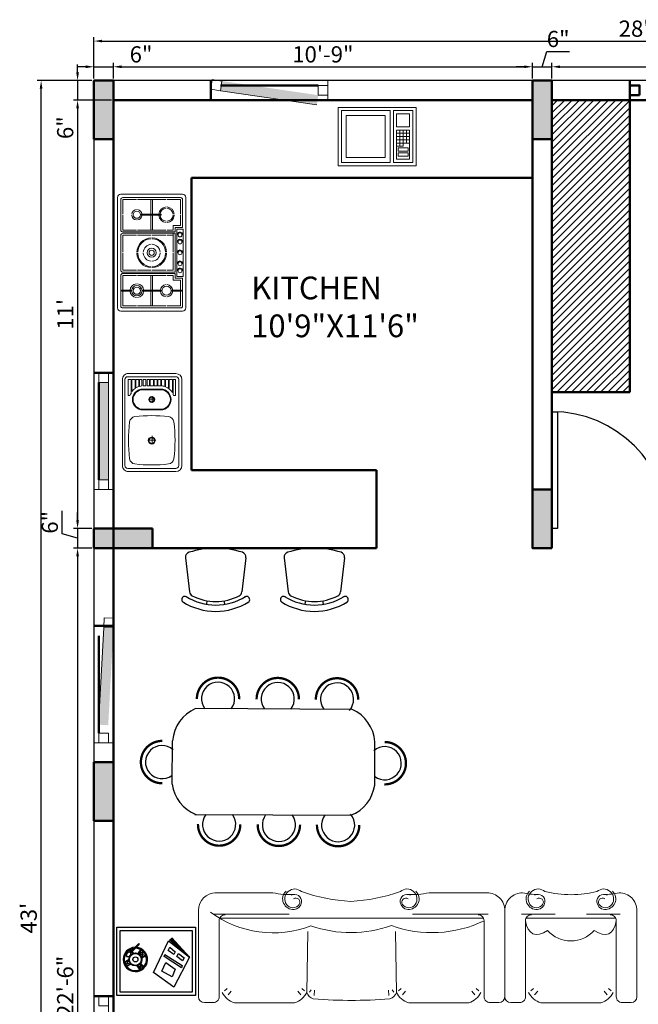
# Model space of a CAD drawing. Units: inches. Extents: x 3064 to 19385, y 846 to 15425.
# Tile 58 of 108: x 6020 to 6210, y 1703 to 2007. Entities that reach past the tile are written whole.
import ezdxf

# ---------------------------------------------------------------- set-up
doc = ezdxf.new("R2010")
doc.units = ezdxf.units.IN
for name, color, linetype, lineweight in [('A-ANNO-DIMS', 2, 'Continuous', 18), ('A-AREA-IDEN', 3, 'Continuous', 18), ('A-COLS', 1, 'Continuous', 35), ('A-DOOR', 3, 'Continuous', 25), ('A-EQPM', 8, 'Continuous', 18), ('A-FLOR-FIXT', 9, 'Continuous', 18), ('A-FURN', 8, 'Continuous', 18), ('A-FURN-PATT', 252, 'Continuous', 13), ('A-GLAZ', 4, 'Continuous', 18), ('A-WALL', 7, 'Continuous', 50), ('C-PROP', 6, 'Continuous', 25)]:
    doc.layers.add(name, color=color, linetype=linetype, lineweight=lineweight)
for name, color, linetype in [('BLO', 135, 'Continuous'), ('FUR', 42, 'Continuous'), ('NOITHAT', 21, 'Continuous'), ('Win', 152, 'Continuous')]:
    doc.layers.add(name, color=color, linetype=linetype)
doc.styles.get("Standard").update_dxf_attribs({"font": 'arial.ttf'})
doc.dimstyles.new('ISO-25', dxfattribs={"dimtxt": 9, "dimasz": 2.5, "dimexe": 1.25, "dimexo": 0.625, "dimtad": 1, "dimdec": 1, "dimlunit": 3, "dimtxsty": 'Standard', "dimcen": 2.5, "dimadec": 0, "dimazin": 0, "dimtfac": 1, "dimtdec": 1, "dimtmove": 0, "dimatfit": 3, "dimfxl": 1, "dimarcsym": 0})

# ---------------------------------------------------------------- blocks, each defined once
blk = doc.blocks.new('*U3')
for p, q in [((0, 0), (0, -6)), ((36, 0), (36, -6))]:
    blk.add_line(p, q)
blk.add_lwpolyline([(0, 0), (0, 36), (1.75, 36), (1.75, 0)], close=True)
blk.add_arc((0, 0), 36, 0, 90)
blk = doc.blocks.new('din')
at = {"layer": 'FUR', "ltscale": 0.25}
for p, q in [((70.23, 15.24), (9.28, 15.24)), ((0, 3.44), (0, -13.56)), ((79.14, 3.44), (79.14, -13.56)), ((8.91, -26.16), (70.23, -26.16))]:
    blk.add_line(p, q, dxfattribs=at)
at = {"layer": 'FUR', "ltscale": 0.25, "const_width": 0.9}
for points in [[(22.5, 19.02, 1.012537), (5.94, 19.02, 1.012537)], [(45.67, 19.02, 1.012537), (29.11, 19.02, 1.012537)], [(69.02, 19.02, 1.012537), (52.46, 19.02, 1.012537)], [(-3.79, 3.1, 1.012537), (-3.79, -13.47, 1.012537)], [(83.08, 3.1, -1.012537), (83.08, -13.47, -1.012537)], [(23.18, -29.95, -1.012537), (6.61, -29.95, -1.012537)], [(46.34, -29.95, -1.012537), (29.78, -29.95, -1.012537)], [(69.7, -29.95, -1.012537), (53.14, -29.95, -1.012537)]]:
    blk.add_lwpolyline(points, format="xyb", dxfattribs=at)
at = {"layer": 'FUR', "ltscale": 0.25}
for centre, radius, start, end in [((14.22, 19.13), 6.48, 323.1301, 221.2163), ((37.39, 19.13), 6.48, 323.1301, 216.8699), ((60.74, 19.13), 6.48, 323.1301, 216.8699), ((14.55, 1.54), 14.67, 111.0491, 172.5731), ((64.59, 1.54), 14.67, 7.4269, 68.9509), ((-3.89, -5.18), 6.48, 53.1301, 311.2163), ((83.18, -5.18), 6.48, 228.7837, 126.8699), ((15.28, -12.21), 15.34, 185.0602, 245.4675), ((63.86, -12.21), 15.34, 294.5325, 354.9398), ((14.89, -30.05), 6.48, 138.7837, 36.8699), ((38.06, -30.05), 6.48, 143.1301, 36.8699), ((61.42, -30.05), 6.48, 143.1301, 36.8699)]:
    blk.add_arc(centre, radius, start, end, dxfattribs=at)
blk = doc.blocks.new('A$C558E769F')
at = {"layer": 'NOITHAT'}
for p, q in [((29.4, 426.4), (61.1, 154.1)), ((508.9, 426.4), (477.2, 154.1)), ((197.1, 55.9), (201.8, 84.2)), ((341.2, 55.9), (336.5, 84.2))]:
    blk.add_line(p, q, dxfattribs=at)
for centre, radius, start, end in [((69.1, 431), 40, 107.02981, 186.63805), ((269.2, -222), 723, 72.97019, 107.02981), ((469.2, 431), 40, 353.36195, 72.97019), ((25.3, 93.7), 25.7, 44.80366, 252.32262), ((269.2, 492.6), 442.6, 237.77056, 302.22944), ((100.8, 158.7), 40, 186.63805, 243.24485), ((269.2, 492.6), 413.9, 243.24485, 296.75515), ((437.5, 158.7), 40, 296.75515, 353.36195), ((513, 93.7), 25.7, 287.67738, 135.19634), ((269.2, 492.6), 492.6, 237.85101, 302.14899)]:
    blk.add_arc(centre, radius, start, end, dxfattribs=at)
blk = doc.blocks.new('sofa-32')
at = {"color": 0, "linetype": 'ByBlock'}
for p, q in [((-0.026, 0.9238), (-0.1, 0.9238)), ((0.657, 0.9252), (0.1531, 0.9252)), ((1.6158, 0.9252), (2.1197, 0.9252)), ((2.3728, 0.9238), (2.2988, 0.9238)), ((-0.15, 0.15), (-0.15, 0.8738)), ((0.024, 0.2361), (0.024, 0.8738)), ((0.05, 0.8375), (0.05, 0.8379)), ((0.1006, 0.8574), (0.1265, 0.8286)), ((0.7096, 0.8574), (0.6837, 0.8286)), ((0.7682, 0.3257), (0.7597, 0.8384)), ((0.7601, 0.8375), (0.7601, 0.8379)), ((0.7823, 0.8346), (0.7966, 0.8162)), ((0.8227, 0.8633), (0.8259, 0.8195)), ((1.4501, 0.8633), (1.447, 0.8195)), ((1.4906, 0.8346), (1.4762, 0.8162)), ((1.5046, 0.3257), (1.5131, 0.8384)), ((1.5127, 0.8375), (1.5127, 0.8379)), ((1.5632, 0.8574), (1.5891, 0.8286)), ((2.1722, 0.8574), (2.1463, 0.8286)), ((2.2228, 0.8375), (2.2228, 0.8379)), ((2.2228, 0.8375), (2.2228, 0.8379)), ((2.2488, 0.2361), (2.2488, 0.8738)), ((2.4228, 0.15), (2.4228, 0.8738)), ((0.0903, 0.8062), (0.0682, 0.8242)), ((0.7199, 0.8062), (0.742, 0.8242)), ((1.5529, 0.8062), (1.5308, 0.8242)), ((2.1825, 0.8062), (2.2046, 0.8242)), ((-0.01, 0.1801), (0.6238, 0.1801)), ((0.0289, 0.2145), (2.2439, 0.2145)), ((2.2948, 0.1801), (1.661, 0.1801)), ((0, 0), (0.4856, 0)), ((2.2848, 0), (1.7991, 0))]:
    blk.add_line(p, q, dxfattribs=at)
at = {"color": 0, "linetype": 'ByBlock', "extrusion": (0, 0, -1)}
for centre, major_axis, start_param, end_param in [((-0.1, 0.8738), (0.0354, 0.0354), 3.926992, 5.497787), ((-0.026, 0.8738), (-0.0354, 0.0354), 0.785398, 2.356196), ((0.1997, 0.7661), (0.1173, 0.1173), 4.372209, 5.213218), ((0.6105, 0.7661), (0.1173, 0.1173), -0.500829, 0.34018), ((1.6624, 0.7661), (0.1173, 0.1173), 4.372209, 5.213218), ((2.0731, 0.7661), (-0.1173, 0.1173), 1.069968, 1.910976), ((2.2988, 0.8738), (-0.0354, 0.0354), 5.497786, 7.068583), ((2.3728, 0.8738), (0.0354, 0.0354), -0.785398, 0.785398), ((0.8378, 0.8143), (-0.0573, 0.0573), 5.78837, 6.779907), ((1.1202, -2.7856), (2.6094, 2.6094), -0.86827, -0.778364), ((1.1526, -2.7856), (2.6094, 2.6094), -0.792432, -0.702526), ((1.435, 0.8143), (-0.0573, 0.0573), 1.074075, 2.065611), ((0.4599, -0.6685), (0.71, 0.71), 5.048761, 5.844539), ((1.1424, -0.6685), (-0.71, 0.71), 0.438646, 1.125824), ((1.7954, -0.5466), (-0.6249, 0.6249), 0.417642, 1.423136), ((0.074, 0.2361), (0.0354, 0.0354), 2.356194, 3.926992), ((2.1988, 0.2361), (0.0354, 0.0354), 0.785397, 2.356194), ((0, 0.15), (0.1061, 0.1061), 2.356194, 3.926992), ((0.6576, 0.0525), (-0.0624, 0.0624), 4.675944, 7.152385), ((0.6708, 0.0524), (-0.059, 0.059), 3.186406, 6.094039), ((0.6552, 0.0629), (0.0458, 0.0458), 4.523242, 6.472337), ((0.6801, 0.0798), (-0.0245, 0.0245), 1.759948, 4.523241), ((0.6592, 0.0712), (-0.0491, 0.0491), 0.8692, 2.230507), ((1.6256, 0.0712), (-0.0491, 0.0491), 5.623477, 6.984784), ((1.614, 0.0524), (0.059, 0.059), 0.189149, 3.096782), ((1.6047, 0.0798), (0.0245, 0.0245), 1.759947, 4.52324), ((1.6295, 0.0629), (0.0458, 0.0458), 4.52324, 6.472335), ((1.6271, 0.0525), (-0.0624, 0.0624), 0.701599, 3.17804), ((2.2728, 0.15), (0.1061, 0.1061), 0.785398, 2.356194), ((0.6324, -0.6613), (-0.479, 0.479), 0.566947, 0.842011), ((0.6701, 0.0726), (0.0414, 0.0414), 0.659711, 2.852687), ((1.2153, -1.3904), (1.0359, 1.0359), 5.158011, 5.447964), ((1.0694, -1.3904), (1.0359, 1.0359), 5.547613, 5.837566), ((1.6147, 0.0726), (-0.0414, 0.0414), 3.430501, 5.623477), ((1.6523, -0.6613), (0.479, 0.479), 5.441177, 5.716241)]:
    blk.add_ellipse(centre, major_axis=major_axis, ratio=1, start_param=start_param, end_param=end_param, dxfattribs=at)
blk = doc.blocks.new('sofa-34')
at = {"color": 0, "linetype": 'ByBlock'}
for p, q in [((-0.026, 0.9238), (-0.1, 0.9238)), ((0.657, 0.9252), (0.1531, 0.9252)), ((0.8361, 0.9238), (0.9101, 0.9238)), ((-0.15, 0.15), (-0.15, 0.8738)), ((0.024, 0.2361), (0.024, 0.8738)), ((0.05, 0.8375), (0.05, 0.8379)), ((0.1006, 0.8574), (0.1265, 0.8286)), ((0.7096, 0.8574), (0.6837, 0.8286)), ((0.7601, 0.8375), (0.7601, 0.8379)), ((0.7602, 0.8375), (0.7601, 0.8379)), ((0.7861, 0.2361), (0.7861, 0.8738)), ((0.9601, 0.15), (0.9601, 0.8738)), ((0.0903, 0.8062), (0.0682, 0.8242)), ((0.7199, 0.8062), (0.742, 0.8242)), ((-0.01, 0.1801), (0.2738, 0.1801)), ((0.0289, 0.2145), (0.7812, 0.2145)), ((0.8201, 0.1801), (0.5364, 0.1801))]:
    blk.add_line(p, q, dxfattribs=at)
blk.add_arc((0.4051, 0.1479), 0.2579, 40.79835, 139.20165, dxfattribs=at)
at = {"color": 0, "linetype": 'ByBlock', "extrusion": (0, 0, -1)}
for centre, major_axis, ratio, start_param, end_param in [((-0.1, 0.8738), (0.0354, 0.0354), 1, 3.926992, 5.497787), ((-0.026, 0.8738), (-0.0354, 0.0354), 1, 0.785398, 2.356196), ((0.1997, 0.7661), (0.1173, 0.1173), 1, 4.372209, 5.213218), ((0.6105, 0.7661), (0.1173, 0.1173), 1, -0.500829, 0.34018), ((0.5004, -0.5869), (-0.4145, 0.931), 0.264583, -0.381915, 0.387685), ((0.074, 0.2361), (-0.0354, 0.0354), 1, 3.926991, 5.497788), ((0, 0.15), (0.1061, 0.1061), 1, 2.356194, 3.926992), ((0.1167, 0.0525), (-0.0624, 0.0624), 1, 4.675944, 7.152385), ((0.1299, 0.0524), (-0.059, 0.059), 1, 3.186406, 6.094039), ((0.1144, 0.0629), (-0.0458, 0.0458), 1, 6.094039, 8.043134), ((0.1392, 0.0798), (0.0245, 0.0245), 1, 0.189152, 2.952444), ((0.1183, 0.0712), (0.0491, 0.0491), 1, -0.701597, 0.659711), ((0.179, -0.6576), (-0.2506, 0.635), 0.885019, 0.124301, 0.339591), ((0.1292, 0.0726), (-0.0414, 0.0414), 1, 2.230507, 4.423483), ((0.3517, -0.5578), (0.7346, 0.1067), 0.76838, 4.597815, 5.20076)]:
    blk.add_ellipse(centre, major_axis=major_axis, ratio=ratio, start_param=start_param, end_param=end_param, dxfattribs=at)
at = {"color": 0, "linetype": 'ByBlock'}
for centre, major_axis, ratio, start_param, end_param in [((0.8361, 0.8738), (0.0354, 0.0354), 1, 0.785398, 2.356196), ((0.9101, 0.8738), (-0.0354, 0.0354), 1, 3.926992, 5.497787), ((0.3097, -0.5869), (0.4145, 0.931), 0.264583, -0.381915, 0.387685), ((0.7361, 0.2361), (0.0354, 0.0354), 1, 3.926991, 5.497788), ((0.6918, 0.0712), (-0.0491, 0.0491), 1, -0.701597, 0.659711), ((0.6802, 0.0524), (0.059, 0.059), 1, 3.186406, 6.094039), ((0.6709, 0.0798), (-0.0245, 0.0245), 1, 0.189152, 2.952444), ((0.6958, 0.0629), (0.0458, 0.0458), 1, 6.094039, 8.043134), ((0.6934, 0.0525), (0.0624, 0.0624), 1, 4.675944, 7.152385), ((0.8101, 0.15), (-0.1061, 0.1061), 1, 2.356194, 3.926992), ((0.6809, 0.0726), (0.0414, 0.0414), 1, 2.230507, 4.423483), ((0.6312, -0.6576), (0.2506, 0.635), 0.885019, 0.124301, 0.339591)]:
    blk.add_ellipse(centre, major_axis=major_axis, ratio=ratio, start_param=start_param, end_param=end_param, dxfattribs=at)
blk = doc.blocks.new('sink 1')
for points in [[(-7.34, 1.48), (-7.34, 22.73)], [(-6.56, 1.48), (-6.56, 22.73)], [(5.86, 24.22), (-5.86, 24.22)], [(6.01, 23.43), (-5.86, 23.43)], [(6.72, 1.48), (6.72, 22.73)], [(7.34, 1.48), (7.34, 22.73)], [(0, 15.39), (0, 17.42)], [(1.09, 16.48), (-0.94, 16.48)], [(-2.09, 8.99), (2.28, 8.99)], [(-2.09, 8.84), (2.28, 8.84)], [(-5.78, 5.39), (-5.78, 5.39)], [(-5.31, 5.39), (-5.31, 5.39)], [(-5.16, 4.92), (-5.16, 4.92)], [(0.78, 6.33), (-0.78, 6.33)], [(0, 5.55), (0, 7.26)], [(5.16, 4.92), (5.16, 4.92)], [(5.94, 5.39), (5.94, 5.39)], [(-5, 1.48), (-5, 4.69)], [(-5, 1.48), (-4.22, 1.48), (-4.22, 3.83)], [(-4.84, 4.45), (-4.84, 4.45)], [(-4.22, 3.83), (-4.22, 3.83)], [(-4.06, 1.48), (-4.06, 3.69)], [(-4.06, 1.48), (-3.28, 1.48), (-3.28, 3.27)], [(-3.91, 3.52), (-3.91, 3.52)], [(-3.28, 3.2), (-3.28, 3.2)], [(-3.12, 3.2), (-3.12, 3.2)], [(-2.34, 3.05), (-2.34, 3.05)], [(-2.19, 3.05), (-2.19, 3.05)], [(-2.09, 3.99), (2.28, 3.99)], [(-2.09, 3.84), (2.28, 3.84)], [(-1.41, 3.05), (-1.41, 3.05)], [(-1.25, 3.05), (-1.25, 3.05)], [(-0.47, 1.48), (-1.25, 1.48), (-1.25, 3.05), (-0.47, 3.05)], [(-0.62, 3.05), (-0.62, 3.05)], [(-0.47, 1.48), (-0.47, 3.05)], [(-0.31, 3.05), (-0.31, 3.05)], [(0.47, 1.48), (-0.31, 1.48), (-0.31, 3.05), (0.47, 3.05)], [(0.31, 3.05), (0.31, 3.05)], [(0.47, 1.48), (0.47, 3.05)], [(0.62, 3.05), (0.62, 3.05)], [(1.25, 3.05), (1.25, 3.05)], [(1.56, 3.05), (1.56, 3.05)], [(2.19, 3.05), (2.19, 3.05)], [(2.5, 3.05), (2.5, 3.05)], [(3.12, 3.2), (3.12, 3.2)], [(3.28, 1.48), (4.06, 1.48), (4.06, 3.57)], [(3.28, 1.48), (3.28, 3.2)], [(3.44, 3.2), (3.44, 3.2)], [(4.06, 3.52), (4.06, 3.52)], [(4.22, 1.48), (4.22, 3.67)], [(4.37, 3.83), (4.37, 3.83)], [(5, 4.45), (5, 4.45)], [(6.01, 0.78), (-5.86, 0.78)], [(5.86, 0), (-5.86, 0)], [(-5.78, 1.48), (-5.78, 1.48)], [(-5.16, 1.48), (-5.16, 1.48)], [(-4.84, 1.48), (-4.84, 1.48)], [(-4.22, 1.48), (-4.22, 1.48)], [(-3.91, 1.48), (-3.91, 1.48)], [(-3.28, 1.48), (-3.28, 1.48)], [(-3.12, 1.48), (-3.12, 1.48)], [(-2.34, 1.48), (-2.34, 1.48)], [(-2.19, 1.48), (-2.19, 1.48)], [(-1.41, 1.48), (-1.41, 1.48)], [(-1.25, 1.48), (-1.25, 1.48)], [(-0.62, 1.48), (-0.62, 1.48)], [(-0.31, 1.48), (-0.31, 1.48)], [(0.31, 1.48), (0.31, 1.48)], [(0.62, 1.48), (0.62, 1.48)], [(1.25, 1.48), (1.25, 1.48)], [(1.56, 1.48), (1.56, 1.48)], [(2.19, 1.48), (2.19, 1.48)], [(2.5, 1.48), (2.5, 1.48)], [(3.12, 1.48), (3.12, 1.48)], [(3.44, 1.48), (3.44, 1.48)], [(4.06, 1.48), (4.06, 1.48)], [(4.37, 1.48), (4.37, 1.48)], [(5, 1.48), (5, 1.48)], [(5.16, 1.48), (5.16, 1.48)], [(5.94, 1.48), (5.94, 1.48)]]:
    blk.add_lwpolyline(points)
for points in [[(-5.16, 4.92), (-5.16, 1.48), (-5.78, 1.48), (-5.78, 5.39), (-5.31, 5.39, -0.068511), (-5.16, 4.92)], [(5.16, 4.92, 0.248301), (5.47, 5.39), (5.94, 5.39), (5.94, 1.48), (5.16, 1.48), (5.16, 4.92)], [(4.06, 3.57, -0.061679), (3.32, 3.22)], [(4.22, 1.48), (5, 1.48), (5, 4.45, -0.083542), (4.22, 3.67, -0.083542)]]:
    blk.add_lwpolyline(points, format="xyb")
for points in [[(-3.12, 3.22), (-3.12, 1.48), (-2.34, 1.48), (-2.34, 3.05, -0.06228)], [(2.5, 3.05), (2.5, 1.48), (3.12, 1.48), (3.12, 3.2, -0.050256)]]:
    blk.add_lwpolyline(points, format="xyb", close=True)
for points in [[(-2.19, 3.05), (-1.41, 3.05), (-1.41, 1.48), (-2.19, 1.48)], [(0.62, 3.05), (1.25, 3.05), (1.25, 1.48), (0.62, 1.48)], [(2.19, 1.48), (2.19, 3.05), (1.56, 3.05), (1.56, 1.48)]]:
    blk.add_lwpolyline(points, close=True)
for centre, radius in [((0.09, 16.57), 0.859), ((0.09, 16.57), 0.703), ((0.09, 6.41), 0.703), ((0.09, 6.41), 0.547)]:
    blk.add_circle(centre, radius)
for centre, radius, start, end in [((-5.86, 22.73), 1.48, 90, 180), ((-5.86, 22.73), 0.703, 90, 180), ((-3.87, 20.82), 1.53, 97.3256, 171.1849), ((0.09, -12.65), 35.23, 83.2159, 96.7841), ((4.06, 20.82), 1.53, 8.8151, 82.6744), ((5.86, 22.73), 1.48, 360, 90), ((6.01, 22.73), 0.703, 0, 90), ((30.19, 16.56), 35.85, 172.7947, 187.4213), ((-30, 16.56), 35.85, 352.5787, 7.2053), ((-3.89, 12.12), 1.48, 187.4212, 263.2159), ((0.09, 45.63), 35.23, 263.2159, 276.7841), ((4.08, 12.12), 1.48, 276.7841, 352.5788), ((-2.1, 6.41), 2.58, 90, 270), ((-2.1, 6.41), 2.42, 90, 270), ((2.28, 6.41), 2.58, 270, 90), ((2.28, 6.41), 2.42, 270, 90), ((-2.15, 6.48), 3.36, 212.1095, 232.0862), ((-2.1, 6.41), 3.36, 234.156, 249.3275), ((2.14, 6.36), 3.36, 289.8633, 290.5971), ((-5.86, 1.48), 1.48, 180, 270), ((-5.86, 1.48), 0.703, 180, 270), ((5.86, 1.48), 1.48, 270, 0), ((6.01, 1.48), 0.703, 270, 360)]:
    blk.add_arc(centre, radius, start, end)
blk = doc.blocks.new('STOVE')
for p, q in [((11.85, 19.7), (11.55, 19.7)), ((11.55, 16.92), (11.55, 19.7)), ((11.85, 16.92), (11.85, 19.7)), ((11.85, 16.92), (11.55, 16.92)), ((-11.85, 13.73), (-11.85, 7.62)), ((-11.85, 13.73), (-11.55, 13.73)), ((-11.55, 13.73), (-11.55, 7.62)), ((11.85, 13.23), (11.55, 13.23)), ((11.55, 13.23), (11.55, 7.57)), ((11.85, 13.23), (11.85, 7.57)), ((-11.85, 10.75), (-16.4, 10.75)), ((-11.85, 10.25), (-16.4, 10.25)), ((-7, 10.75), (-11.55, 10.75)), ((-7, 10.25), (-11.55, 10.25)), ((7, 10.75), (11.55, 10.75)), ((7, 10.25), (11.55, 10.25)), ((11.85, 10.75), (16.4, 10.75)), ((11.85, 10.25), (16.4, 10.25)), ((-11.85, 7.62), (-11.55, 7.62)), ((11.85, 7.57), (11.55, 7.57)), ((-7, 3.9), (-8.4, 3.9)), ((-7.8, 3.3), (-7.8, 1)), ((-6.4, 3.3), (-7.8, 3.3)), ((-5.4, 3.9), (-6, 3.9)), ((-5.4, 3.9), (-0.15, 3.9)), ((0.15, 3.9), (5.4, 3.9)), ((6.4, 3.3), (7.8, 3.3)), ((7, 3.9), (8.4, 3.9)), ((7.8, 3.3), (7.8, 1)), ((8.4, 3.9), (8.4, 1.6)), ((11.85, 4.28), (11.55, 4.28)), ((11.55, 4.28), (11.55, 1.3)), ((11.85, 4.28), (11.85, 1.3)), ((7.3, 2.8), (-7.3, 2.8)), ((-7.3, 2.8), (-7.3, 0.8)), ((7.3, 0.8), (-7.3, 0.8)), ((7.3, 2.8), (7.3, 0.8)), ((11.85, 1.3), (11.55, 1.3))]:
    blk.add_line(p, q)
for points in [[(-17, 21), (17, 21, -0.414214), (18, 20), (18, 1, -0.414214), (17, 0), (-17, 0, -0.414214), (-18, 1), (-18, 20, -0.414214)], [(6, 3.3), (-6, 3.3), (-6, 19.4, -0.414214), (-5.4, 20), (5.4, 20, -0.414214), (6, 19.4)]]:
    blk.add_lwpolyline(points, format="xyb", close=True)
for points in [[(-7.8, 1), (-16.4, 1, -0.414214), (-17, 1.6), (-17, 19.4, -0.414214), (-16.4, 20), (-7, 20, -0.414214), (-6.4, 19.4), (-6.4, 3.3)], [(6.4, 19.4, -0.414214), (7, 20), (16.4, 20, -0.414214), (17, 19.4), (17, 1.6, -0.414214), (16.4, 1), (7.8, 1)]]:
    blk.add_lwpolyline(points, format="xyb")
for points in [[(-16.4, 15.22), (-16.4, 19.4), (-11.85, 19.4)], [(-11.55, 19.4), (-7, 19.4), (-7, 15.22)], [(-5.4, 15.22), (-5.4, 19.4), (-0.15, 19.4)], [(0.15, 19.4), (5.4, 19.4), (5.4, 15.22)], [(6.4, 3.3), (6.4, 19.4)], [(7, 15.22), (7, 19.4), (11.55, 19.4)], [(11.85, 19.4), (16.4, 19.4), (16.4, 15.22)], [(-16.4, 6.08), (-16.4, 14.92)], [(-7, 14.92), (-7, 6.08)], [(-5.4, 10.65), (-5.4, 14.92)], [(5.4, 14.92), (5.4, 10.65)], [(7, 6.08), (7, 14.92)], [(16.4, 14.92), (16.4, 6.08)], [(-5.4, 6.08), (-5.4, 10.35)], [(5.4, 10.35), (5.4, 6.08)], [(-11.85, 1.6), (-16.4, 1.6), (-16.4, 5.77)], [(-8.4, 3.9), (-8.4, 1.6), (-11.55, 1.6)], [(-7, 5.77), (-7, 3.9)], [(-5.4, 3.9), (-5.4, 5.77)], [(5.4, 5.77), (5.4, 3.9)], [(7, 3.9), (7, 5.77)], [(16.4, 5.77), (16.4, 1.6), (11.85, 1.6)], [(11.55, 1.6), (8.4, 1.6)]]:
    blk.add_lwpolyline(points)
for centre, radius in [((-11.7, 15.07), 1.1), ((11.7, 15.07), 1.6), ((11.7, 15.07), 1.1), ((0, 10.5), 1.4), ((0, 10.5), 0.8), ((11.7, 5.93), 1.4), ((-5.49, 1.8), 0.6), ((-3.3, 1.8), 0.6), ((0, 1.8), 0.6), ((3.39, 1.8), 0.6), ((5.57, 1.8), 0.6)]:
    blk.add_circle(centre, radius)
for centre, radius, start, end in [((-11.7, 15.07), 1.6, 95.3794, 174.6206), ((-11.7, 15.07), 1.6, 5.3794, 84.6206), ((11.7, 15.07), 2.1, 94.096, 175.904), ((11.7, 15.07), 2.1, 4.096, 85.904), ((-11.7, 15.07), 1.6, 185.3794, 264.6206), ((-11.7, 15.07), 1.6, 275.3794, 354.6206), ((0, 10.5), 4.6, 91.8687, 178.1313), ((0, 10.5), 4.3, 91.9991, 178.0009), ((0, 10.5), 2.6, 93.3074, 176.6926), ((0, 10.5), 4.6, 1.8687, 88.1313), ((0, 10.5), 4.3, 1.9991, 88.0009), ((0, 10.5), 2.6, 3.3074, 86.6926), ((11.7, 15.07), 2.1, 184.096, 265.904), ((11.7, 15.07), 2.1, 274.096, 355.904), ((0, 10.5), 4.6, 181.8687, 268.1313), ((0, 10.5), 4.3, 181.9991, 268.0009), ((0, 10.5), 2.6, 183.3074, 266.6926), ((0, 10.5), 4.6, 271.8687, 358.1313), ((0, 10.5), 4.3, 271.9991, 358.0009), ((0, 10.5), 2.6, 273.3074, 356.6926), ((-11.7, 5.93), 2.4, 93.5833, 176.4167), ((-11.7, 5.93), 2, 94.3012, 175.6988), ((-11.7, 5.93), 2.4, 3.5833, 86.4167), ((-11.7, 5.93), 2, 4.3012, 85.6988), ((11.7, 5.93), 1.9, 94.5281, 175.4719), ((11.7, 5.93), 1.9, 4.5281, 85.4719), ((-11.7, 5.93), 2.4, 183.5833, 266.4167), ((-11.7, 5.93), 2, 184.3012, 265.6988), ((-11.7, 5.93), 2.4, 273.5833, 356.4167), ((-11.7, 5.93), 2, 274.3012, 355.6988), ((11.7, 5.93), 1.9, 184.5281, 265.4719), ((11.7, 5.93), 1.9, 274.5281, 355.4719), ((-5.49, 1.8), 0.846, 89.9979, 270), ((-3.3, 1.8), 0.846, 89.9979, 270), ((0, 1.8), 0.846, 89.9979, 270), ((3.39, 1.8), 0.846, 89.9979, 270), ((5.57, 1.8), 0.846, 89.9979, 270)]:
    blk.add_arc(centre, radius, start, end)
blk = doc.blocks.new('Microwave')
for p, q in [((18, 10), (22, 10)), ((19, 7), (19, 11)), ((20, 11), (20, 7)), ((21, 7), (21, 11)), ((22, 9), (18, 9)), ((18, 8), (22, 8)), ((22, 7), (18, 7)), ((19, 6), (19, 7)), ((20, 7), (20, 6)), ((20, 6), (18, 6))]:
    blk.add_line(p, q)
for points in [[(0, 0), (0, 18), (24, 18), (24, 0)], [(1, 1), (1, 17), (16, 17), (16, 1)], [(2.5, 2.5), (2.5, 15.5), (14.5, 15.5), (14.5, 2.5)], [(17, 1), (17, 17), (23, 17), (23, 1)], [(18, 12), (18, 16), (22, 16), (22, 12)], [(18, 2), (18, 11), (22, 11), (22, 2)], [(18.5, 4.5), (18.5, 5.5), (21.5, 5.5), (21.5, 4.5)], [(18.5, 3), (18.5, 4), (21.5, 4), (21.5, 3)]]:
    blk.add_lwpolyline(points, close=True)
blk = doc.blocks.new('*D384')
at = {"layer": 'A-ANNO-DIMS', "color": 0, "lineweight": -2, "transparency": 16777216}
for p, q in [((6042.49, 1988.61), (6042.49, 1993.49)), ((6048.49, 1988.61), (6048.49, 1993.49)), ((6039.99, 1992.24), (6037.49, 1992.24)), ((6042.49, 1992.24), (6048.49, 1992.24)), ((6050.99, 1992.24), (6060.52, 1992.24))]:
    blk.add_line(p, q, dxfattribs=at)
at = {"layer": 'A-ANNO-DIMS', "color": 0, "transparency": 16777216}
for points in [[(6039.99, 1992.66), (6039.99, 1991.83), (6042.49, 1992.24)], [(6050.99, 1992.66), (6050.99, 1991.83), (6048.49, 1992.24)]]:
    blk.add_solid(points, dxfattribs=at)
at = {"layer": 'Defpoints', "color": 0, "transparency": 16777216}
for p in [(6048.49, 1992.24), (6042.49, 1987.99), (6048.49, 1987.99)]:
    blk.add_point(p, dxfattribs=at)
at = {"layer": 'A-ANNO-DIMS', "color": 0, "transparency": 16777216, "insert": (6057, 1995.42), "char_height": 5, "attachment_point": 5}
blk.add_mtext('6"', dxfattribs=at)
blk = doc.blocks.new('*D385')
at = {"layer": 'A-ANNO-DIMS', "color": 0, "lineweight": -2, "transparency": 16777216}
for p, q in [((6048.49, 1988.61), (6048.49, 1993.49)), ((6177.49, 1988.61), (6177.49, 1993.49)), ((6050.99, 1992.24), (6174.99, 1992.24))]:
    blk.add_line(p, q, dxfattribs=at)
at = {"layer": 'A-ANNO-DIMS', "color": 0, "transparency": 16777216}
for points in [[(6050.99, 1992.66), (6050.99, 1991.83), (6048.49, 1992.24)], [(6174.99, 1992.66), (6174.99, 1991.83), (6177.49, 1992.24)]]:
    blk.add_solid(points, dxfattribs=at)
at = {"layer": 'Defpoints', "color": 0, "transparency": 16777216}
for p in [(6177.49, 1992.24), (6048.49, 1987.99), (6177.49, 1987.99)]:
    blk.add_point(p, dxfattribs=at)
at = {"layer": 'A-ANNO-DIMS', "color": 0, "transparency": 16777216, "insert": (6112.99, 1995.42), "char_height": 5, "attachment_point": 5}
blk.add_mtext('10\'-9"', dxfattribs=at)
blk = doc.blocks.new('*D386')
at = {"layer": 'A-ANNO-DIMS', "color": 0, "lineweight": -2, "transparency": 16777216}
for p, q in [((6180.49, 1992.24), (6181.91, 1996.98)), ((6181.91, 1996.98), (6188.94, 1996.98)), ((6177.49, 1988.61), (6177.49, 1993.49)), ((6183.49, 1988.61), (6183.49, 1993.49)), ((6174.99, 1992.24), (6172.49, 1992.24)), ((6177.49, 1992.24), (6183.49, 1992.24)), ((6177.49, 1992.24), (6183.49, 1992.24)), ((6185.99, 1992.24), (6188.49, 1992.24))]:
    blk.add_line(p, q, dxfattribs=at)
at = {"layer": 'A-ANNO-DIMS', "color": 0, "transparency": 16777216}
for points in [[(6174.99, 1992.66), (6174.99, 1991.83), (6177.49, 1992.24)], [(6185.99, 1992.66), (6185.99, 1991.83), (6183.49, 1992.24)]]:
    blk.add_solid(points, dxfattribs=at)
at = {"layer": 'Defpoints', "color": 0, "transparency": 16777216}
for p in [(6183.49, 1992.24), (6177.49, 1987.99), (6183.49, 1987.99)]:
    blk.add_point(p, dxfattribs=at)
at = {"layer": 'A-ANNO-DIMS', "color": 0, "transparency": 16777216, "insert": (6185.43, 2000.16), "char_height": 5, "attachment_point": 5}
blk.add_mtext('6"', dxfattribs=at)
blk = doc.blocks.new('*D387')
at = {"layer": 'A-ANNO-DIMS', "color": 0, "lineweight": -2, "transparency": 16777216}
for p, q in [((6183.49, 1988.61), (6183.49, 1993.49)), ((6378.49, 1988.61), (6378.49, 1993.49)), ((6185.99, 1992.24), (6375.99, 1992.24))]:
    blk.add_line(p, q, dxfattribs=at)
at = {"layer": 'A-ANNO-DIMS', "color": 0, "transparency": 16777216}
for points in [[(6185.99, 1992.66), (6185.99, 1991.83), (6183.49, 1992.24)], [(6375.99, 1992.66), (6375.99, 1991.83), (6378.49, 1992.24)]]:
    blk.add_solid(points, dxfattribs=at)
at = {"layer": 'Defpoints', "color": 0, "transparency": 16777216}
for p in [(6378.49, 1992.24), (6183.49, 1987.99), (6378.49, 1987.99)]:
    blk.add_point(p, dxfattribs=at)
at = {"layer": 'A-ANNO-DIMS', "color": 0, "transparency": 16777216, "insert": (6280.99, 1995.42), "char_height": 5, "attachment_point": 5}
blk.add_mtext('16\'-3"', dxfattribs=at)
blk = doc.blocks.new('*D389')
at = {"layer": 'A-ANNO-DIMS', "color": 0, "lineweight": -2, "transparency": 16777216}
for p, q in [((6037.46, 1990.49), (6037.46, 1992.99)), ((6041.87, 1987.99), (6036.21, 1987.99)), ((6037.46, 1987.99), (6037.46, 1981.99)), ((6047.87, 1981.99), (6036.21, 1981.99)), ((6037.46, 1979.49), (6037.46, 1969.96))]:
    blk.add_line(p, q, dxfattribs=at)
at = {"layer": 'A-ANNO-DIMS', "color": 0, "transparency": 16777216}
for points in [[(6037.05, 1990.49), (6037.88, 1990.49), (6037.46, 1987.99)], [(6037.05, 1979.49), (6037.88, 1979.49), (6037.46, 1981.99)]]:
    blk.add_solid(points, dxfattribs=at)
at = {"layer": 'Defpoints', "color": 0, "transparency": 16777216}
for p in [(6042.49, 1987.99), (6037.46, 1981.99), (6048.49, 1981.99)]:
    blk.add_point(p, dxfattribs=at)
at = {"layer": 'A-ANNO-DIMS', "color": 0, "transparency": 16777216, "insert": (6034.29, 1973.48), "char_height": 5, "attachment_point": 5, "rotation": 90}
blk.add_mtext('6"', dxfattribs=at)
blk = doc.blocks.new('*D390')
at = {"layer": 'A-ANNO-DIMS', "color": 0, "lineweight": -2, "transparency": 16777216}
for p, q in [((6047.87, 1981.99), (6036.21, 1981.99)), ((6037.46, 1979.49), (6037.46, 1852.49)), ((6041.87, 1849.99), (6036.21, 1849.99))]:
    blk.add_line(p, q, dxfattribs=at)
at = {"layer": 'A-ANNO-DIMS', "color": 0, "transparency": 16777216}
for points in [[(6037.05, 1979.49), (6037.88, 1979.49), (6037.46, 1981.99)], [(6037.05, 1852.49), (6037.88, 1852.49), (6037.46, 1849.99)]]:
    blk.add_solid(points, dxfattribs=at)
at = {"layer": 'Defpoints', "color": 0, "transparency": 16777216}
for p in [(6048.49, 1981.99), (6037.46, 1849.99), (6042.49, 1849.99)]:
    blk.add_point(p, dxfattribs=at)
at = {"layer": 'A-ANNO-DIMS', "color": 0, "transparency": 16777216, "insert": (6034.33, 1915.99), "char_height": 5, "attachment_point": 5, "rotation": 90}
blk.add_mtext("11'", dxfattribs=at)
blk = doc.blocks.new('*D391')
at = {"layer": 'A-ANNO-DIMS', "color": 0, "lineweight": -2, "transparency": 16777216}
for p, q in [((6032.72, 1848.41), (6032.72, 1855.44)), ((6037.46, 1852.49), (6037.46, 1854.99)), ((6037.46, 1846.99), (6032.72, 1848.41)), ((6041.87, 1849.99), (6036.21, 1849.99)), ((6037.46, 1849.99), (6037.46, 1843.99)), ((6037.46, 1849.99), (6037.46, 1843.99)), ((6041.87, 1843.99), (6036.21, 1843.99)), ((6037.46, 1841.49), (6037.46, 1838.99))]:
    blk.add_line(p, q, dxfattribs=at)
at = {"layer": 'A-ANNO-DIMS', "color": 0, "transparency": 16777216}
for points in [[(6037.05, 1852.49), (6037.88, 1852.49), (6037.46, 1849.99)], [(6037.05, 1841.49), (6037.88, 1841.49), (6037.46, 1843.99)]]:
    blk.add_solid(points, dxfattribs=at)
at = {"layer": 'Defpoints', "color": 0, "transparency": 16777216}
for p in [(6042.49, 1849.99), (6037.46, 1843.99), (6042.49, 1843.99)]:
    blk.add_point(p, dxfattribs=at)
at = {"layer": 'A-ANNO-DIMS', "color": 0, "transparency": 16777216, "insert": (6029.55, 1851.92), "char_height": 5, "attachment_point": 5, "rotation": 90}
blk.add_mtext('6"', dxfattribs=at)
blk = doc.blocks.new('*D380')
at = {"layer": 'A-ANNO-DIMS', "color": 0, "lineweight": -2, "transparency": 16777216}
for p, q in [((6041.87, 1843.99), (6036.21, 1843.99)), ((6037.46, 1841.49), (6037.46, 1576.49)), ((6047.87, 1573.99), (6036.21, 1573.99))]:
    blk.add_line(p, q, dxfattribs=at)
at = {"layer": 'A-ANNO-DIMS', "color": 0, "transparency": 16777216}
for points in [[(6037.05, 1841.49), (6037.88, 1841.49), (6037.46, 1843.99)], [(6037.05, 1576.49), (6037.88, 1576.49), (6037.46, 1573.99)]]:
    blk.add_solid(points, dxfattribs=at)
at = {"layer": 'Defpoints', "color": 0, "transparency": 16777216}
for p in [(6042.49, 1843.99), (6037.46, 1573.99), (6048.49, 1573.99)]:
    blk.add_point(p, dxfattribs=at)
at = {"layer": 'A-ANNO-DIMS', "color": 0, "transparency": 16777216, "insert": (6034.29, 1708.99), "char_height": 5, "attachment_point": 5, "rotation": 90}
blk.add_mtext('22\'-6"', dxfattribs=at)
blk = doc.blocks.new('*D354')
at = {"layer": 'A-ANNO-DIMS', "color": 0, "lineweight": -2, "transparency": 16777216}
for p, q in [((6041.87, 1987.99), (6024.98, 1987.99)), ((6026.23, 1474.49), (6026.23, 1985.49)), ((6041.87, 1471.99), (6024.98, 1471.99))]:
    blk.add_line(p, q, dxfattribs=at)
at = {"layer": 'A-ANNO-DIMS', "color": 0, "transparency": 16777216}
for points in [[(6025.81, 1985.49), (6026.64, 1985.49), (6026.23, 1987.99)], [(6025.81, 1474.49), (6026.64, 1474.49), (6026.23, 1471.99)]]:
    blk.add_solid(points, dxfattribs=at)
at = {"layer": 'Defpoints', "color": 0, "transparency": 16777216}
for p in [(6026.23, 1987.99), (6042.49, 1987.99), (6042.49, 1471.99)]:
    blk.add_point(p, dxfattribs=at)
at = {"layer": 'A-ANNO-DIMS', "color": 0, "transparency": 16777216, "insert": (6023.05, 1729.99), "char_height": 5, "attachment_point": 5, "rotation": 90}
blk.add_mtext("43'", dxfattribs=at)
blk = doc.blocks.new('*D378')
at = {"layer": 'A-ANNO-DIMS', "color": 0, "lineweight": -2, "transparency": 16777216}
for p, q in [((6042.49, 1988.61), (6042.49, 2001.41)), ((6044.99, 2000.16), (6381.99, 2000.16)), ((6384.49, 1988.61), (6384.49, 2001.41))]:
    blk.add_line(p, q, dxfattribs=at)
at = {"layer": 'A-ANNO-DIMS', "color": 0, "transparency": 16777216}
for points in [[(6044.99, 2000.58), (6044.99, 1999.75), (6042.49, 2000.16)], [(6381.99, 2000.58), (6381.99, 1999.75), (6384.49, 2000.16)]]:
    blk.add_solid(points, dxfattribs=at)
at = {"layer": 'Defpoints', "color": 0, "transparency": 16777216}
for p in [(6384.49, 2000.16), (6042.49, 1987.99), (6384.49, 1987.99)]:
    blk.add_point(p, dxfattribs=at)
at = {"layer": 'A-ANNO-DIMS', "color": 0, "transparency": 16777216, "insert": (6213.49, 2003.34), "char_height": 5, "attachment_point": 5}
blk.add_mtext('28\'-6"', dxfattribs=at)
blk = doc.blocks.new('ST1')
at = {"layer": 'BLO'}
for p, q in [((2.87, 1.65), (2.87, 24.72)), ((2.87, 24.72), (22.87, 24.72)), ((3.87, 2.65), (3.87, 23.72)), ((3.87, 23.72), (21.87, 23.72)), ((21.87, 23.72), (21.87, 2.65)), ((22.87, 24.72), (22.87, 1.65)), ((22.87, 1.65), (2.87, 1.65)), ((21.87, 2.65), (3.87, 2.65))]:
    blk.add_line(p, q, dxfattribs=at)
at = {"layer": 'Win'}
for p, q in [((11.4, 21.86), (12.09, 20.65)), ((11.51, 21.94), (12.19, 20.74)), ((11.57, 21.85), (13.19, 21.3)), ((12.55, 22.44), (12.13, 20.85)), ((12.55, 22.44), (13.25, 21.19)), ((12.69, 22.48), (13.4, 21.2)), ((14.51, 20.87), (14.54, 20.9)), ((14.64, 20.77), (14.67, 20.79)), ((15.43, 20.61), (15.22, 19.97)), ((15.22, 19.97), (15.71, 20.33)), ((15.27, 19.81), (15.82, 20.21)), ((15.37, 21.5), (15.64, 21.7)), ((15.41, 20.64), (17.8, 18.17)), ((15.46, 21.36), (15.76, 21.58)), ((15.54, 20.8), (16.34, 20.79)), ((15.54, 20.77), (18.02, 18.4)), ((15.76, 21.58), (15.55, 20.96)), ((17.88, 18.31), (15.58, 20.6)), ((15.87, 20.45), (16.34, 20.79)), ((15.99, 20.33), (16.41, 20.64)), ((10.46, 17.93), (11.6, 18.76)), ((10.53, 17.78), (11.65, 18.59)), ((10.53, 17.78), (12.23, 17.8)), ((11.59, 18.54), (11.11, 16.99)), ((11.11, 16.99), (12.23, 17.8)), ((11.23, 16.87), (12.37, 17.7)), ((13.9, 17.44), (14.58, 16.23)), ((14.03, 17.48), (14.71, 16.28)), ((14.09, 17.38), (15.67, 16.91)), ((15.04, 18.04), (14.71, 16.28)), ((14.97, 18.16), (15.67, 16.91)), ((15, 18.22), (15.87, 17.69)), ((15.13, 18.43), (16.01, 17.9)), ((15.14, 18.13), (15.77, 17.01)), ((5.28, 8.07), (9.58, 13.93)), ((8.3, 8.54), (10.02, 11.57)), ((9.58, 13.93), (18.91, 9.59)), ((10.02, 11.57), (12.5, 10.4)), ((12.5, 10.4), (10.58, 7.59)), ((10.98, 5.74), (14.34, 10.89)), ((14.87, 10.68), (11.67, 5.58)), ((18.91, 9.59), (14.09, 3.45)), ((14.09, 3.45), (19.17, 9.31)), ((14.09, 3.45), (19.44, 9.01)), ((14.09, 3.45), (19.64, 8.8)), ((14.34, 10.89), (14.87, 10.68)), ((14.86, 8.07), (16.06, 9.73)), ((17.01, 9.23), (15.7, 7.6)), ((16.06, 9.73), (17.01, 9.23)), ((14.09, 3.45), (5.28, 8.07)), ((10.58, 7.59), (8.3, 8.54)), ((13.06, 5.5), (14.27, 7.16)), ((15.21, 6.66), (13.91, 5.03)), ((14.09, 3.45), (19.77, 8.63)), ((14.27, 7.16), (15.21, 6.66)), ((15.7, 7.6), (14.86, 8.07)), ((11.67, 5.58), (10.98, 5.74)), ((13.91, 5.03), (13.06, 5.5))]:
    blk.add_line(p, q, dxfattribs=at)
for radius in [1.91, 1.75, 0.74]:
    blk.add_circle((13.43, 19.29), radius, dxfattribs=at)
for centre, radius, start, end in [((13.43, 19.29), 3.56, 1.5005, 355.5882), ((13.43, 19.29), 3.27, 6.8421, 0.252), ((15.21, 21.57), 0.956, 171.718, 281.8824), ((14.47, 21.69), 0.203, 96.3605, 174.3012), ((14.6, 20.95), 0.956, 349.0729, 98.9437), ((15.51, 20.66), 0.106, 78.1124, 194.2793), ((15.97, 17.77), 0.128, 220.7943, 60.0122), ((17.91, 18.29), 0.161, 227.8642, 43.7153)]:
    blk.add_arc(centre, radius, start, end, dxfattribs=at)
blk = doc.blocks.new('WIN-900-A')
h = blk.add_hatch(color=256)
h.dxf.hatch_style = 1
h.paths.add_polyline_path([(33, 0), (33, 3), (3, 3), (3, 0)])
blk.add_line((3, 0), (33, 0))
blk.add_lwpolyline([(3, 0), (0, 0), (0, 3), (3, 3)], close=True)
blk = doc.blocks.new('WIN-900')
blk.add_line((0, 0), (30, 0))
blk.add_lwpolyline([(30, 0), (30, 3), (33, 3), (33, 0)], close=True)
blk = doc.blocks.new('WIN-1900')
blk.add_line((3, 0), (3, 66))
blk.add_lwpolyline([(3, 66), (0, 66), (0, 69), (3, 69)], close=True)

msp = doc.modelspace()

# ---------------------------------------------------------------- hatches: boundary and pattern name
at = {"layer": 'A-COLS'}
h = msp.add_hatch(color=256, dxfattribs=at)
h.dxf.hatch_style = 1
h.paths.add_polyline_path([(6042.49, 1969.99), (6048.49, 1969.99), (6048.49, 1987.99), (6042.49, 1987.99)])
h = msp.add_hatch(color=256, dxfattribs=at)
h.dxf.hatch_style = 1
h.paths.add_polyline_path([(6177.49, 1969.99), (6183.49, 1969.99), (6183.49, 1987.99), (6177.49, 1987.99)])
h = msp.add_hatch(color=256, dxfattribs=at)
h.dxf.hatch_style = 1
h.paths.add_polyline_path([(6177.49, 1843.99), (6183.49, 1843.99), (6183.49, 1861.99), (6177.49, 1861.99)])
h = msp.add_hatch(color=256, dxfattribs=at)
h.dxf.hatch_style = 1
h.paths.add_polyline_path([(6060.49, 1843.99), (6060.49, 1849.99), (6042.49, 1849.99), (6042.49, 1843.99)])
h = msp.add_hatch(color=256, dxfattribs=at)
h.dxf.hatch_style = 1
h.paths.add_polyline_path([(6042.49, 1759.99), (6048.49, 1759.99), (6048.49, 1777.99), (6042.49, 1777.99)])
at = {"layer": 'A-FURN-PATT'}
h = msp.add_hatch(dxfattribs=at)
h.set_pattern_fill('ANSI31', color=256, scale=0.5)
h.set_pattern_definition([(45, (726.825, 591.649), (-1.122532, 1.122532), [])])
h.paths.add_polyline_path([(6207.49, 1981.99), (6183.49, 1981.99), (6183.49, 1969.99), (6183.49, 1891.99), (6207.49, 1891.99)])
at = {"layer": 'A-GLAZ'}
h = msp.add_hatch(color=256, dxfattribs=at)
h.dxf.hatch_style = 1
h.paths.add_polyline_path([(6043.99, 1864.99), (6046.99, 1864.99), (6046.99, 1894.99), (6043.99, 1894.99)])

# ---------------------------------------------------------------- linework, layer by layer
for p, q in [((6114.49, 1987.99), (6114.49, 1981.99)), ((6042.49, 1861.99), (6048.49, 1861.99)), ((6042.49, 1783.99), (6048.49, 1783.99))]:
    msp.add_line(p, q, dxfattribs=at)
for points in [[(6114.49, 1983.49), (6111.49, 1983.49), (6111.49, 1986.49), (6114.49, 1986.49)], [(6046.99, 1861.99), (6043.99, 1861.99), (6043.99, 1864.99), (6046.99, 1864.99)], [(6046.99, 1783.99), (6043.99, 1783.99), (6043.99, 1786.99), (6046.99, 1786.99)]]:
    msp.add_lwpolyline(points, close=True, dxfattribs=at)
at = {"layer": 'A-WALL'}
for p, q in [((6078.49, 1987.99), (6078.49, 1981.99)), ((6207.49, 1987.99), (6207.49, 1981.99)), ((6081.49, 1986.49), (6111.49, 1986.49)), ((6177.49, 1981.99), (6048.49, 1981.99)), ((6048.49, 1981.99), (6048.49, 1573.99)), ((6177.49, 1981.99), (6177.49, 1843.99)), ((6378.49, 1981.99), (6183.49, 1981.99)), ((6183.49, 1981.99), (6183.49, 1843.99)), ((6207.49, 1981.99), (6207.49, 1891.99)), ((6177.49, 1957.99), (6072.49, 1957.99)), ((6072.49, 1957.99), (6072.49, 1867.99)), ((6042.49, 1897.99), (6048.49, 1897.99)), ((6043.99, 1894.99), (6043.99, 1864.99)), ((6207.49, 1891.99), (6183.49, 1891.99)), ((6072.49, 1867.99), (6129.49, 1867.99)), ((6129.49, 1867.99), (6129.49, 1843.99)), ((6048.49, 1843.99), (6129.49, 1843.99)), ((6183.49, 1843.99), (6177.49, 1843.99)), ((6042.49, 1819.99), (6048.49, 1819.99)), ((6043.99, 1816.99), (6043.99, 1786.99)), ((6048.49, 1705.99), (6042.49, 1705.99))]:
    msp.add_line(p, q, dxfattribs=at)
for points in [[(6048.49, 1969.99), (6048.49, 1987.99), (6042.49, 1987.99), (6042.49, 1969.99)], [(6183.49, 1969.99), (6183.49, 1987.99), (6177.49, 1987.99), (6177.49, 1969.99)], [(6210.49, 1983.49), (6207.49, 1983.49), (6207.49, 1986.49), (6210.49, 1986.49)], [(6183.49, 1843.99), (6183.49, 1861.99), (6177.49, 1861.99), (6177.49, 1843.99)], [(6060.49, 1849.99), (6042.49, 1849.99), (6042.49, 1843.99), (6060.49, 1843.99)], [(6048.49, 1759.99), (6048.49, 1777.99), (6042.49, 1777.99), (6042.49, 1759.99)]]:
    msp.add_lwpolyline(points, close=True, dxfattribs=at)
at = {"layer": 'C-PROP'}
for p, q in [((6384.49, 1987.99), (6042.49, 1987.99)), ((6042.49, 1987.99), (6042.49, 1471.99))]:
    msp.add_line(p, q, dxfattribs=at)

# ---------------------------------------------------------------- block references
at = {"layer": 'A-DOOR'}
msp.add_blockref('*U3', (6183.49, 1849.99), dxfattribs=at)
at = {"layer": 'A-EQPM'}
msp.add_blockref('Microwave', (6117.7, 1961.75), dxfattribs=at)
at = {"layer": 'A-EQPM', "xscale": -1, "rotation": 90}
msp.add_blockref('STOVE', (6070.78, 1934.96), dxfattribs=at)
at = {"layer": 'A-FLOR-FIXT', "xscale": 1.24732326381372, "yscale": 1.24732326381372, "zscale": 1.24732326381372, "rotation": 180}
msp.add_blockref('sink 1', (6060.41, 1897.75), dxfattribs=at)
at = {"layer": 'A-FURN', "xscale": 0.0387879515044038, "yscale": 0.0387879515044038, "zscale": 0.0387879515044038}
for p in [(6069.56, 1824.49), (6099.92, 1824.49)]:
    msp.add_blockref('A$C558E769F', p, dxfattribs=at)
at = {"layer": 'A-FURN'}
for name, p, xscale, yscale, zscale, rotation in [('din', (6128.95, 1773.65), 0.787402, 0.787402, 0.787402, 179.7134895170222), ('sofa-32', (6163.49, 1737.83), 36.66436083614781, 36.66436083614781, 36.66436083614781, 180), ('sofa-34', (6174.49, 1737.83), -36.66436083614781, 36.66436083614781, 36.66436083614781, 180), ('ST1', (6075.54, 1703.14), 1.051988476719542, 1.051988476719542, 1.051988476719542, 90)]:
    msp.add_blockref(name, p, dxfattribs=dict(at, xscale=xscale, yscale=yscale, zscale=zscale, rotation=rotation))
at = {"layer": 'A-GLAZ'}
for name, p, rotation in [('WIN-900-A', (6078.48, 1985.32), 351.6350998303226), ('WIN-900', (6046.99, 1864.99), 90.00000000000244), ('WIN-900-A', (6045.67, 1822.53), 266.917355118037)]:
    msp.add_blockref(name, p, dxfattribs=dict(at, rotation=rotation))
msp.add_blockref('WIN-1900', (6043.99, 1636.99), dxfattribs=at)

# ---------------------------------------------------------------- texts
at = {"layer": 'A-AREA-IDEN', "insert": (6090.91, 1927.61), "char_height": 7, "attachment_point": 1}
msp.add_mtext_dynamic_manual_height_columns('KITCHEN\\P10\'9"X11\'6"', width=67.5924, gutter_width=12.5, heights=[0], dxfattribs=at)

# ---------------------------------------------------------------- dimensions: what is measured, and where the dimension line sits
at = {"layer": 'A-ANNO-DIMS'}
for base, p1, p2, override, picture, middle in [((6384.49, 2000.16), (6042.49, 1987.99), (6384.49, 1987.99), {"dimtxt": 5, "dimclrd": 0, "dimclre": 0, "dimclrt": 0}, '*D378', (6213.49, 2003.34)), ((6183.49, 1992.24), (6177.49, 1987.99), (6183.49, 1987.99), {"dimtxt": 5, "dimclrd": 0, "dimclre": 0, "dimclrt": 0, "dimtmove": 1}, '*D386', (6182.54, 2000.16)), ((6048.49, 1992.24), (6042.49, 1987.99), (6048.49, 1987.99), {"dimtxt": 5, "dimclrd": 0, "dimclre": 0, "dimclrt": 0}, '*D384', (6057, 1995.42)), ((6177.49, 1992.24), (6048.49, 1987.99), (6177.49, 1987.99), {"dimtxt": 5, "dimclrd": 0, "dimclre": 0, "dimclrt": 0, "dimtmove": 1}, '*D385', (6112.99, 1995.42)), ((6378.49, 1992.24), (6183.49, 1987.99), (6378.49, 1987.99), {"dimtxt": 5, "dimclrd": 0, "dimclre": 0, "dimclrt": 0, "dimtmove": 1}, '*D387', (6280.99, 1995.42))]:
    dim = msp.add_linear_dim(base=base, p1=p1, p2=p2, dimstyle='ISO-25', override=override, dxfattribs=at)
    dim.commit()
    dim.dimension.update_dxf_attribs({"geometry": picture, "text_midpoint": middle})
for base, p1, p2, override, picture, middle in [((6037.46, 1981.99), (6042.49, 1987.99), (6048.49, 1981.99), {"dimtxt": 5, "dimclrd": 0, "dimclre": 0, "dimclrt": 0}, '*D389', (6034.29, 1973.48)), ((6026.23, 1987.99), (6042.49, 1471.99), (6042.49, 1987.99), {"dimtxt": 5, "dimclrd": 0, "dimclre": 0, "dimclrt": 0}, '*D354', (6023.05, 1729.99)), ((6037.46, 1849.99), (6048.49, 1981.99), (6042.49, 1849.99), {"dimtxt": 5, "dimclrd": 0, "dimclre": 0, "dimclrt": 0, "dimtmove": 1}, '*D390', (6034.33, 1915.99)), ((6037.46, 1843.99), (6042.49, 1849.99), (6042.49, 1843.99), {"dimtxt": 5, "dimclrd": 0, "dimclre": 0, "dimclrt": 0, "dimtmove": 1}, '*D391', (6029.55, 1849.04)), ((6037.46, 1573.99), (6042.49, 1843.99), (6048.49, 1573.99), {"dimtxt": 5, "dimclrd": 0, "dimclre": 0, "dimclrt": 0, "dimtmove": 1}, '*D380', (6034.29, 1708.99))]:
    dim = msp.add_linear_dim(base=base, p1=p1, p2=p2, angle=90, dimstyle='ISO-25', override=override, dxfattribs=at)
    dim.commit()
    dim.dimension.update_dxf_attribs({"geometry": picture, "text_midpoint": middle})

doc.saveas('drawing.dxf')
